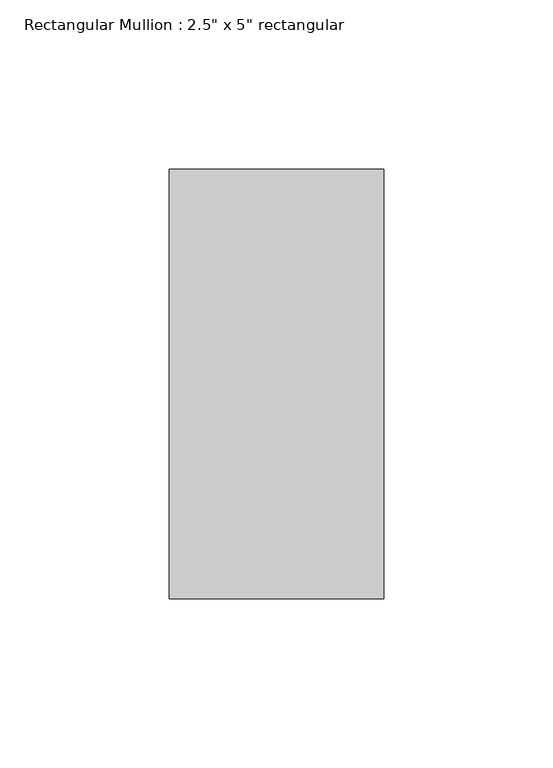
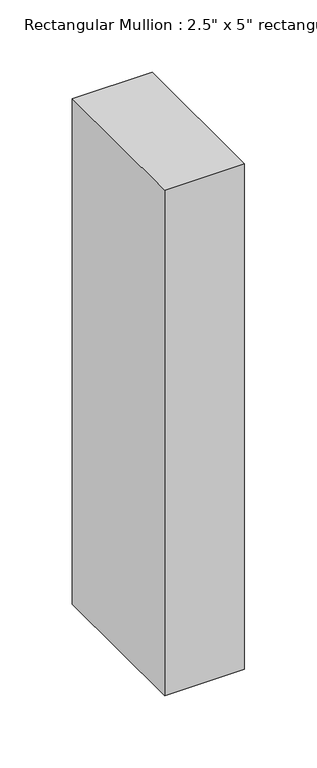
"""IFC4 building model written with IfcOpenShell, lengths in millimetres: member geometry."""

from ifc_helpers import new_model, si_unit, frame, origin, place, context, project, spatial, polyline, outline, extrude, source, transform, mapped, element, save


def member_84b97a81(model_context):
    return source(origin(), model_context, "Body", "SweptSolid", [
        extrude(outline(polyline([(0.0, 63.5), (0.0, -63.5), (-63.5, -63.5), (-63.5, 63.5), (0.0, 63.5)])), frame((0.0, 0.0, -425.45), z_axis=(0.0, 0.0, 1.0), x_axis=(1.0, 0.0, 0.0)), (0.0, 0.0, 1.0), 425.45),
    ])


if __name__ == "__main__":
    model = new_model("IFC4")
    model_context = context("Model", 3, world=origin())
    ifc_project = project(units=[si_unit("LENGTHUNIT", "METRE", prefix="MILLI")], contexts=[model_context])
    site = spatial("IfcSite", under=ifc_project)
    building = spatial("IfcBuilding", under=site)
    placement = place(None, origin())
    member_shape = member_84b97a81(model_context)
    element("IfcMember", 1, ObjectType="Rectangular Mullion : 2.5\" x 5\" rectangular", at=placement, inside=building, context=model_context, shape_type="MappedRepresentation", body=[
        mapped(member_shape, transform((0.0, 0.0, 0.0), x_axis=(1.0, 0.0, 0.0), y_axis=(0.0, 1.0, 0.0), z_axis=(0.0, 0.0, 1.0))),
    ])
    save(model, "model.ifc")

# Revit data of these elements
# Type "Rectangular Mullion : 2.5\" x 5\" rectangular"
#   built-in parameter 1007304 = 0.416667 (stored number, unit not read)
#   built-in parameter 1007301 = 0.104167 (stored number, unit not read)
#   built-in parameter 1007300 = 0.104167 (stored number, unit not read)
# Element 1 (IfcMember, "Rectangular Mullion : 2.5\" x 5\" rectangular")
#   Materials on its faces: "Aluminum"
# Materials
#   "Aluminum": class "Metal", colour RGB 247 247 247, transparency 0, Description = "Aluminum 6061", Cost = 0
